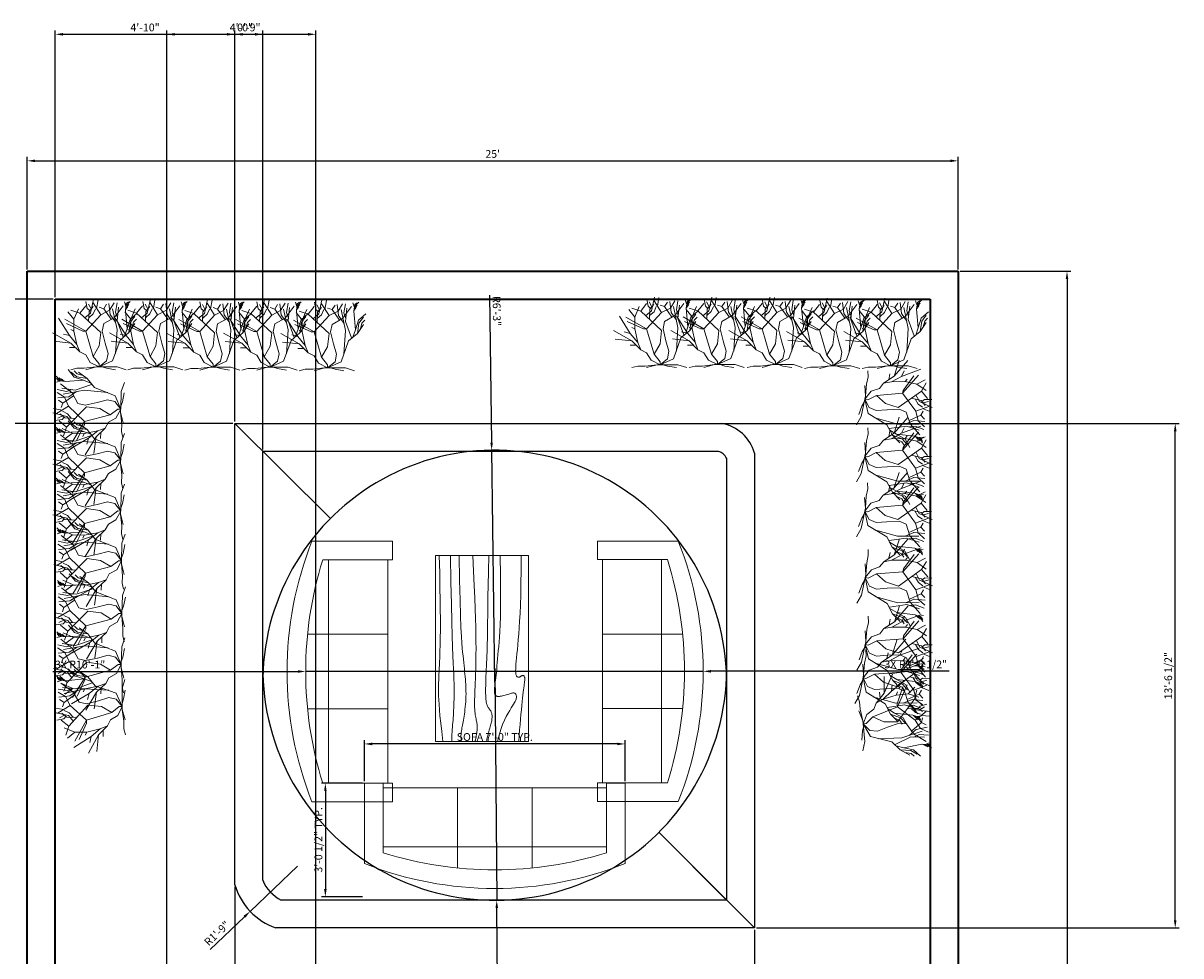
# Model space of a CAD drawing. Units: inches. Extents: x 2318 to 3542, y 1525 to 2117.
# Tile 6 of 6: x 3169 to 3542, y 1816 to 2117. Entities that reach past the tile are written whole.
import ezdxf

# ---------------------------------------------------------------- set-up
doc = ezdxf.new("R2010")
doc.units = ezdxf.units.IN
for name, color, linetype, lineweight in [('A-ANNO-DIMS', 2, 'Continuous', 18), ('A-FLOR', 7, 'Continuous', 25), ('A-FURN', 8, 'Continuous', 18), ('A-WALL', 7, 'Continuous', 35), ('L-PLNT', 94, 'Continuous', 13)]:
    doc.layers.add(name, color=color, linetype=linetype, lineweight=lineweight)
doc.styles.get("Standard").update_dxf_attribs({"font": 'arial.ttf'})
doc.dimstyles.new('ISO-25', dxfattribs={"dimtxt": 2.5, "dimasz": 2.5, "dimexe": 1.25, "dimexo": 0.625, "dimtad": 1, "dimdec": 0, "dimlunit": 3, "dimtxsty": 'Standard', "dimcen": 2.5, "dimadec": 0, "dimazin": 0, "dimtfac": 1, "dimtdec": 0, "dimtmove": 0, "dimatfit": 3, "dimfxl": 1, "dimarcsym": 0})

# ---------------------------------------------------------------- blocks, each defined once
blk = doc.blocks.new('*D19')
at = {"layer": 'A-ANNO-DIMS', "color": 0, "lineweight": -2, "transparency": 16777216}
for p, q in [((3170.43, 2037.71), (3170.43, 2073.97)), ((3172.93, 2072.72), (3467.93, 2072.72)), ((3470.43, 2037.71), (3470.43, 2073.97))]:
    blk.add_line(p, q, dxfattribs=at)
at = {"layer": 'A-ANNO-DIMS', "color": 0, "transparency": 16777216}
for points in [[(3172.93, 2073.14), (3172.93, 2072.3), (3170.43, 2072.72)], [(3467.93, 2073.14), (3467.93, 2072.3), (3470.43, 2072.72)]]:
    blk.add_solid(points, dxfattribs=at)
at = {"layer": 'Defpoints', "color": 0, "transparency": 16777216}
for p in [(3470.43, 2072.72), (3170.43, 2037.09), (3470.43, 2037.09)]:
    blk.add_point(p, dxfattribs=at)
at = {"layer": 'A-ANNO-DIMS', "color": 0, "transparency": 16777216, "insert": (3320.43, 2074.62), "char_height": 2.5, "attachment_point": 5}
blk.add_mtext("25'", dxfattribs=at)
blk = doc.blocks.new('*D20')
at = {"layer": 'A-ANNO-DIMS', "color": 0, "lineweight": -2, "transparency": 16777216}
for p, q in [((3471.06, 2037.09), (3506.78, 2037.09)), ((3505.53, 2034.59), (3505.53, 1559.59)), ((3471.06, 1557.09), (3506.78, 1557.09))]:
    blk.add_line(p, q, dxfattribs=at)
at = {"layer": 'A-ANNO-DIMS', "color": 0, "transparency": 16777216}
for points in [[(3505.11, 2034.59), (3505.94, 2034.59), (3505.53, 2037.09)], [(3505.11, 1559.59), (3505.94, 1559.59), (3505.53, 1557.09)]]:
    blk.add_solid(points, dxfattribs=at)
at = {"layer": 'Defpoints', "color": 0, "transparency": 16777216}
for p in [(3470.43, 2037.09), (3470.43, 1557.09), (3505.53, 1557.09)]:
    blk.add_point(p, dxfattribs=at)
at = {"layer": 'A-ANNO-DIMS', "color": 0, "transparency": 16777216, "insert": (3503.63, 1797.09), "char_height": 2.5, "attachment_point": 5, "rotation": 90}
blk.add_mtext("40'", dxfattribs=at)
blk = doc.blocks.new('*U22')
for p, q in [((-290.3982, 464.5406), (-265.6078, 577.8246)), ((-240.792, 502.285), (-228.3968, 573.8368)), ((-426.72, 414.528), (-475.488, 475.488)), ((-377.952, 463.296), (-451.104, 487.68)), ((-426.72, 414.528), (-390.144, 499.872)), ((-377.952, 463.296), (-329.184, 524.256)), ((-316.7634, 502.285), (-327.6092, 559.9176)), ((-296.5958, 484.4034), (-316.7634, 502.285)), ((-286.512, 498.3226), (-307.4416, 538.0736)), ((-305.8922, 396.9512), (-302.7934, 478.4344)), ((-302.7934, 478.4344), (-270.256, 518.1854)), ((-268.7066, 458.5716), (-250.0884, 500.3038)), ((-207.264, 451.104), (-268.224, 548.64)), ((-182.88, 499.872), (-219.456, 512.064)), ((-207.264, 451.104), (-134.112, 487.68)), ((-182.88, 499.872), (-158.496, 536.448)), ((-121.92, 414.528), (-182.88, 499.872)), ((-129.1844, 450.6214), (-140.0302, 542.036)), ((-134.112, 487.68), (-97.536, 548.64)), ((-73.152, 329.184), (-109.728, 499.872)), ((-97.536, 426.72), (-24.384, 524.256)), ((-85.7758, 472.4908), (-73.3552, 548.005)), ((-73.152, 402.336), (-60.96, 512.064)), ((-12.9032, 555.9552), (-2.0574, 522.1732)), ((-5.1562, 486.3846), (2.5908, 542.036)), ((8.7884, 335.3562), (-5.1562, 486.3846)), ((-3.6068, 492.3536), (14.986, 518.1854)), ((-0.508, 508.254), (22.7584, 536.067)), ((1.0414, 526.1356), (35.1536, 559.9176)), ((2.5908, 542.036), (21.209, 555.9552)), ((-463.296, 280.416), (-552.577, 423.037)), ((-329.184, 316.992), (-499.872, 414.528)), ((-426.72, 316.992), (-426.72, 414.528)), ((-207.264, 304.8), (-377.952, 463.296)), ((-338.455, 424.7896), (-290.3982, 464.5406)), ((-329.184, 316.992), (-207.264, 451.104)), ((-304.3428, 426.7708), (-268.7066, 458.5716)), ((-182.88, 377.952), (-97.536, 426.72)), ((-85.7758, 389.001), (-129.1844, 452.6026)), ((-70.2564, 426.7708), (-85.7758, 472.4908)), ((-24.384, 268.224), (-73.152, 402.336)), ((8.7884, 335.3562), (33.6042, 412.8516)), ((24.384, 304.8), (36.576, 390.144)), ((33.6042, 412.8516), (92.5068, 464.5406)), ((36.576, 390.144), (73.152, 438.912)), ((48.768, 341.376), (60.96, 390.144)), ((60.96, 390.144), (85.344, 414.528)), ((-451.104, 219.456), (-601.0402, 303.8094)), ((-463.296, 280.416), (-512.064, 292.608)), ((-353.568, 316.992), (-487.68, 377.952)), ((-426.72, 316.992), (-451.104, 329.184)), ((-402.336, 207.264), (-426.72, 316.992)), ((-329.184, 316.992), (-353.568, 316.992)), ((-268.224, 109.728), (-329.184, 316.992)), ((-219.456, 195.072), (-207.264, 304.8)), ((-195.072, 316.992), (-182.88, 377.952)), ((-170.688, 219.456), (-195.072, 316.992)), ((-85.344, 134.112), (-73.152, 329.184)), ((-48.768, 243.84), (24.384, 304.8)), ((-12.192, 274.32), (8.7884, 335.3562)), ((24.384, 304.8), (73.152, 377.952)), ((-451.104, 219.456), (-587.4512, 234.2388)), ((-402.336, 207.264), (-463.296, 280.416)), ((-377.952, 146.304), (-451.104, 219.456)), ((-377.952, 146.304), (-402.336, 207.264)), ((-268.224, 109.728), (-219.456, 195.072)), ((-146.304, 134.112), (-170.688, 219.456)), ((-109.728, 73.152), (-48.768, 243.84)), ((-414.528, 182.88), (-463.296, 182.88)), ((-329.184, 121.92), (-377.952, 146.304)), ((-292.608, 60.96), (-329.184, 121.92)), ((-219.456, 48.768), (-268.224, 109.728)), ((-158.496, 73.152), (-146.304, 134.112)), ((-402.336, 12.192), (-451.104, 0)), ((-341.376, 12.192), (-402.336, 12.192)), ((-243.84, 24.384), (-341.376, 12.192)), ((-243.84, 24.384), (-329.184, 0)), ((-219.456, 24.384), (-292.608, 60.96)), ((-243.84, 24.384), (-195.072, 24.384)), ((-219.456, 24.384), (-109.728, 73.152)), ((-219.456, 24.384), (-158.496, 73.152)), ((-219.456, 24.384), (-219.456, 48.768)), ((-219.456, 24.384), (-73.152, 24.384)), ((-195.072, 24.384), (-158.496, 12.192)), ((-158.496, 12.192), (-85.344, 0)), ((-73.152, 24.384), (0, 0))]:
    blk.add_line(p, q)
blk = doc.blocks.new('Table - Rectangular Woodgrain 60 x 30 in.')
for p, q in [((0, 0), (0, -30)), ((60, 0), (0, 0)), ((60, -30), (60, 0)), ((0, -30), (60, -30))]:
    blk.add_line(p, q)
for points in [[(0, -2.4), (4.8155, -2.418), (9.0302, -2.4688), (12.709, -2.5477), (15.9167, -2.65), (18.7181, -2.7711), (21.1781, -2.9063), (23.3616, -3.0508), (25.3333, -3.2), (27.1477, -3.3495), (28.8172, -3.4958), (30.3437, -3.636), (31.7291, -3.7667), (32.9756, -3.8849), (34.0849, -3.9875), (35.059, -4.0714), (35.9, -4.1334), (36.6114, -4.1711), (37.2041, -4.1854), (37.6906, -4.1779), (38.0833, -4.15), (38.3948, -4.1034), (38.6375, -4.0396), (38.8239, -3.9602), (38.9666, -3.8667), (39.0764, -3.7608), (39.1573, -3.6448), (39.2116, -3.521), (39.2416, -3.3917), (39.2498, -3.2593), (39.2385, -3.1261), (39.21, -2.9944), (39.1666, -2.8667), (39.111, -2.7447), (39.0468, -2.6281), (38.978, -2.5163), (38.9083, -2.4083), (38.8418, -2.3035), (38.7823, -2.201), (38.7337, -2.1001), (38.7, -2), (38.6844, -1.9003), (38.6875, -1.8021), (38.7094, -1.707), (38.75, -1.6167), (38.8094, -1.5326), (38.8875, -1.4563), (38.9844, -1.3893), (39.1, -1.3333), (39.2351, -1.2896), (39.3937, -1.2583), (39.5804, -1.2396), (39.8, -1.2333), (40.057, -1.2396), (40.3562, -1.2583), (40.7023, -1.2896), (41.1, -1.3333), (41.5547, -1.3895), (42.0755, -1.4573), (42.6721, -1.5361), (43.3542, -1.625), (44.1316, -1.7233), (45.014, -1.8302), (46.0114, -1.9449), (47.1333, -2.0667), (48.3862, -2.1947), (49.7625, -2.3281), (51.2513, -2.4663), (52.8416, -2.6083), (54.5226, -2.7535), (56.2833, -2.9011), (58.1127, -3.0501), (60, -3.2)], [(0, -9.2), (6.5759, -9.0858), (11.9385, -9.0365), (16.2527, -9.0418), (19.6833, -9.0917), (22.3952, -9.1759), (24.5531, -9.2844), (26.322, -9.4069), (27.8666, -9.5333), (29.3241, -9.6553), (30.7203, -9.7719), (32.0532, -9.8837), (33.3208, -9.9917), (34.5213, -10.0965), (35.6526, -10.199), (36.7128, -10.2999), (37.7, -10.4), (38.6129, -10.4996), (39.4531, -10.5969), (40.223, -10.6895), (40.925, -10.775), (41.5613, -10.8512), (42.1344, -10.9156), (42.6465, -10.966), (43.1, -11), (43.4976, -11.0158), (43.8437, -11.0136), (44.143, -10.9942), (44.4, -10.9583), (44.6195, -10.9069), (44.8062, -10.8406), (44.9648, -10.7603), (45.1, -10.6667), (45.2155, -10.5598), (45.3114, -10.4365), (45.3871, -10.2929), (45.4416, -10.125), (45.4743, -9.929), (45.4844, -9.7011), (45.4709, -9.4371), (45.4333, -9.1333), (45.3716, -8.7883), (45.2896, -8.4104), (45.1919, -8.0107), (45.0833, -7.6), (44.9685, -7.1893), (44.8521, -6.7896), (44.7388, -6.4117), (44.6333, -6.0667), (44.54, -5.7628), (44.4614, -5.4979), (44.4001, -5.2675), (44.3583, -5.0667), (44.3384, -4.8909), (44.3427, -4.7354), (44.3736, -4.5956), (44.4333, -4.4667), (44.5236, -4.3453), (44.6427, -4.2333), (44.7884, -4.1339), (44.9583, -4.05), (45.1501, -3.9849), (45.3614, -3.9417), (45.59, -3.9234), (45.8333, -3.9333), (46.0915, -3.9749), (46.3734, -4.0531), (46.6906, -4.1736), (47.0542, -4.3417), (47.4756, -4.5629), (47.9661, -4.8427), (48.5372, -5.1866), (49.2, -5.6), (49.9676, -6.0844), (50.8594, -6.625), (51.8965, -7.2031), (53.1, -7.8), (54.491, -8.3969), (56.0906, -8.975), (57.9199, -9.5156), (60, -10)], [(0, -12.8), (5.1847, -12.9322), (9.6213, -13.0323), (13.3963, -13.1059), (16.5958, -13.1583), (19.3063, -13.1952), (21.614, -13.2219), (23.6054, -13.2439), (25.3666, -13.2667), (26.9728, -13.2947), (28.4531, -13.3281), (29.8256, -13.3663), (31.1083, -13.4083), (32.3191, -13.4535), (33.476, -13.501), (34.597, -13.5501), (35.7, -13.6), (36.7984, -13.6497), (37.8875, -13.6979), (38.9578, -13.743), (40, -13.7833), (41.0047, -13.8174), (41.9625, -13.8438), (42.864, -13.8607), (43.7, -13.8667), (44.4631, -13.8604), (45.1552, -13.8417), (45.7801, -13.8104), (46.3416, -13.7667), (46.8439, -13.7104), (47.2906, -13.6417), (47.6858, -13.5604), (48.0333, -13.4667), (48.3375, -13.3608), (48.6042, -13.2448), (48.8396, -13.121), (49.05, -12.9917), (49.2417, -12.8593), (49.4208, -12.7261), (49.5937, -12.5944), (49.7667, -12.4667), (49.9452, -12.3451), (50.1323, -12.2313), (50.3303, -12.1268), (50.5416, -12.0333), (50.7686, -11.9524), (51.0135, -11.8854), (51.2788, -11.8341), (51.5666, -11.8), (51.8785, -11.7843), (52.2116, -11.7865), (52.562, -11.8059), (52.926, -11.8417), (53.2998, -11.8931), (53.6795, -11.9594), (54.0614, -12.0397), (54.4416, -12.1333), (54.8223, -12.2401), (55.2293, -12.3625), (55.6942, -12.5037), (56.2489, -12.6667), (56.9251, -12.8547), (57.7545, -13.0708), (58.7689, -13.3182), (60, -13.6)], [(0, -18), (5.124, -17.7273), (9.6609, -17.5057), (13.6705, -17.3303), (17.2125, -17.1958), (20.3467, -17.0973), (23.1328, -17.0297), (25.6307, -16.9878), (27.9, -16.9667), (29.9928, -16.9617), (31.9302, -16.9703), (33.7254, -16.9907), (35.3917, -17.0208), (36.9423, -17.0588), (38.3906, -17.1026), (39.7499, -17.1503), (41.0333, -17.2), (42.2519, -17.2496), (43.4073, -17.2969), (44.4986, -17.3395), (45.525, -17.375), (46.4858, -17.4012), (47.3802, -17.4156), (48.2074, -17.416), (48.9667, -17.4), (49.6583, -17.3662), (50.2872, -17.3167), (50.8595, -17.2547), (51.3812, -17.1833), (51.8584, -17.1057), (52.2971, -17.025), (52.7034, -16.9443), (53.0833, -16.8667), (53.443, -16.7951), (53.789, -16.7313), (54.128, -16.6768), (54.4666, -16.6334), (54.8115, -16.6024), (55.1693, -16.5854), (55.5465, -16.5841), (55.95, -16.6), (56.3828, -16.6337), (56.8346, -16.6823), (57.2915, -16.7418), (57.7396, -16.8084), (58.165, -16.878), (58.5539, -16.9469), (58.8924, -17.0111), (59.1666, -17.0667), (59.3679, -17.1107), (59.5078, -17.1438), (59.6032, -17.1675), (59.6708, -17.1833), (59.7275, -17.193), (59.7901, -17.1979), (59.8753, -17.1998), (60, -17.2)], [(0, -22.4), (8.0098, -22.2501), (14.4094, -22.1011), (19.4168, -21.9535), (23.25, -21.8083), (26.1269, -21.6663), (28.2656, -21.5281), (29.884, -21.3947), (31.2, -21.2667), (32.3967, -21.1448), (33.5172, -21.0292), (34.5697, -20.9198), (35.5625, -20.8167), (36.5037, -20.7198), (37.4015, -20.6292), (38.2642, -20.5448), (39.1, -20.4667), (39.9164, -20.3951), (40.7187, -20.3313), (41.5117, -20.2768), (42.3, -20.2333), (43.0883, -20.2024), (43.8812, -20.1854), (44.6836, -20.1841), (45.5, -20.2), (46.3328, -20.234), (47.1747, -20.2844), (48.0163, -20.3488), (48.8479, -20.425), (49.66, -20.5106), (50.4429, -20.6031), (51.1872, -20.7004), (51.8833, -20.8), (52.5246, -20.8999), (53.1166, -20.9995), (53.6681, -21.0983), (54.1875, -21.1958), (54.6834, -21.2919), (55.1646, -21.3859), (55.6394, -21.4777), (56.1167, -21.5667), (56.6028, -21.6515), (57.0961, -21.7266), (57.5929, -21.7852), (58.0896, -21.8208), (58.5823, -21.8268), (59.0674, -21.7964), (59.5412, -21.723), (60, -21.6)], [(0, -25.2), (8.6355, -25.0504), (15.7026, -24.9031), (21.4049, -24.7606), (25.9458, -24.625), (29.529, -24.4988), (32.3578, -24.3844), (34.6359, -24.284), (36.5667, -24.2), (38.3213, -24.1341), (39.9417, -24.0854), (41.437, -24.0523), (42.8167, -24.0333), (44.0901, -24.0268), (45.2667, -24.0313), (46.3557, -24.0451), (47.3667, -24.0667), (48.309, -24.0947), (49.1928, -24.1287), (50.0284, -24.168), (50.826, -24.2125), (51.5959, -24.2617), (52.3483, -24.3151), (53.0935, -24.3725), (53.8417, -24.4334), (54.6009, -24.497), (55.3699, -24.561), (56.1454, -24.6226), (56.9239, -24.6792), (57.7021, -24.7279), (58.4764, -24.7662), (59.2435, -24.7911), (60, -24.8)], [(0, -28.8), (5.6867, -28.6681), (10.45, -28.5698), (14.407, -28.5012), (17.675, -28.4584), (20.3711, -28.4374), (22.6125, -28.4344), (24.5164, -28.4455), (26.2, -28.4667), (27.762, -28.4947), (29.2276, -28.5281), (30.6033, -28.5663), (31.8958, -28.6084), (33.1118, -28.6535), (34.2578, -28.7011), (35.3405, -28.7501), (36.3666, -28.8), (37.3443, -28.8497), (38.288, -28.8974), (39.2137, -28.9412), (40.1375, -28.9792), (41.0753, -29.0093), (42.0432, -29.0297), (43.0572, -29.0384), (44.1333, -29.0333), (45.2936, -29.0114), (46.5843, -28.9641), (48.0579, -28.8816), (49.7666, -28.7542), (51.7629, -28.5721), (54.0989, -28.3255), (56.8272, -28.0048), (60, -27.6)]]:
    blk.add_lwpolyline(points)
blk = doc.blocks.new('Sofa - Roundback 7 ft.')
for p, q in [((-12.00002, -32.4421), (-12.00003, -6.5971)), ((11.99997, -32.4421), (11.99998, -6.5971)), ((-36.000027, -34), (-36.000027, -11.4696)), ((-35.999844, -13.3819), (35.9998, -13.3819)), ((35.99998, -34), (35.99998, -11.4696)), ((-36.000027, -32.4421), (35.99998, -32.4421))]:
    blk.add_line(p, q)
for points in [[(-36.000027, -34), (-42.000027, -34), (-42.000027, -8)], [(41.99998, -8), (41.99998, -34), (35.99998, -34)]]:
    blk.add_lwpolyline(points)
for centre, radius, start, end in [((0, -114.25), 114.25, 68.43141, 111.5686), ((-0.00001, -127.1968), 121.1968, 72.72033, 107.2797)]:
    blk.add_arc(centre, radius, start, end)
blk = doc.blocks.new('*D38')
at = {"layer": 'A-ANNO-DIMS', "color": 0, "lineweight": -2, "transparency": 16777216}
for p, q in [((3279.1, 1872.73), (3279.1, 1885.95)), ((3360.6, 1884.7), (3281.6, 1884.7)), ((3363.1, 1872.73), (3363.1, 1885.95))]:
    blk.add_line(p, q, dxfattribs=at)
at = {"layer": 'A-ANNO-DIMS', "color": 0, "transparency": 16777216}
for points in [[(3281.6, 1885.12), (3281.6, 1884.28), (3279.1, 1884.7)], [(3360.6, 1885.12), (3360.6, 1884.28), (3363.1, 1884.7)]]:
    blk.add_solid(points, dxfattribs=at)
at = {"layer": 'Defpoints', "color": 0, "transparency": 16777216}
for p in [(3279.1, 1884.7), (3279.1, 1872.1), (3363.1, 1872.1)]:
    blk.add_point(p, dxfattribs=at)
at = {"layer": 'A-ANNO-DIMS', "color": 0, "transparency": 16777216, "insert": (3321.1, 1886.62), "char_height": 2.5, "attachment_point": 5}
blk.add_mtext('SOFA 7\'-0" TYP.', dxfattribs=at)
blk = doc.blocks.new('*D39')
at = {"layer": 'A-ANNO-DIMS', "color": 0, "lineweight": -2, "transparency": 16777216}
for p, q in [((3278.47, 1872.1), (3265.25, 1872.1)), ((3266.5, 1869.6), (3266.5, 1837.93)), ((3278.47, 1835.43), (3265.25, 1835.43))]:
    blk.add_line(p, q, dxfattribs=at)
at = {"layer": 'A-ANNO-DIMS', "color": 0, "transparency": 16777216}
for points in [[(3266.08, 1869.6), (3266.91, 1869.6), (3266.5, 1872.1)], [(3266.08, 1837.93), (3266.91, 1837.93), (3266.5, 1835.43)]]:
    blk.add_solid(points, dxfattribs=at)
at = {"layer": 'Defpoints', "color": 0, "transparency": 16777216}
for p in [(3279.1, 1872.1), (3266.5, 1835.43), (3279.1, 1835.43)]:
    blk.add_point(p, dxfattribs=at)
at = {"layer": 'A-ANNO-DIMS', "color": 0, "transparency": 16777216, "insert": (3264.58, 1853.77), "char_height": 2.5, "attachment_point": 5, "rotation": 90}
blk.add_mtext('3\'-0 1/2" TYP.', dxfattribs=at)
blk = doc.blocks.new('*D53')
at = {"layer": 'A-ANNO-DIMS', "color": 0, "lineweight": -2, "transparency": 16777216}
for p, q in [((3237.33, 1838.64), (3237.33, 1529.19)), ((3404.83, 1824.73), (3404.83, 1529.19)), ((3239.83, 1530.44), (3402.33, 1530.44))]:
    blk.add_line(p, q, dxfattribs=at)
at = {"layer": 'A-ANNO-DIMS', "color": 0, "transparency": 16777216}
for points in [[(3239.83, 1530.86), (3239.83, 1530.02), (3237.33, 1530.44)], [(3402.33, 1530.86), (3402.33, 1530.02), (3404.83, 1530.44)]]:
    blk.add_solid(points, dxfattribs=at)
at = {"layer": 'Defpoints', "color": 0, "transparency": 16777216}
for p in [(3237.33, 1839.27), (3404.83, 1825.36), (3404.83, 1530.44)]:
    blk.add_point(p, dxfattribs=at)
at = {"layer": 'A-ANNO-DIMS', "color": 0, "transparency": 16777216, "insert": (3321.08, 1532.36), "char_height": 2.5, "attachment_point": 5}
blk.add_mtext('13\'-11 1/2"', dxfattribs=at)
blk = doc.blocks.new('*D54')
at = {"layer": 'A-ANNO-DIMS', "color": 0, "lineweight": -2, "transparency": 16777216}
for p, q in [((3237.96, 1988.05), (3541.66, 1988.05)), ((3540.41, 1827.86), (3540.41, 1985.55)), ((3405.46, 1825.36), (3541.66, 1825.36))]:
    blk.add_line(p, q, dxfattribs=at)
at = {"layer": 'A-ANNO-DIMS', "color": 0, "transparency": 16777216}
for points in [[(3539.99, 1985.55), (3540.82, 1985.55), (3540.41, 1988.05)], [(3539.99, 1827.86), (3540.82, 1827.86), (3540.41, 1825.36)]]:
    blk.add_solid(points, dxfattribs=at)
at = {"layer": 'Defpoints', "color": 0, "transparency": 16777216}
for p in [(3237.33, 1988.05), (3540.41, 1988.05), (3404.83, 1825.36)]:
    blk.add_point(p, dxfattribs=at)
at = {"layer": 'A-ANNO-DIMS', "color": 0, "transparency": 16777216, "insert": (3538.49, 1906.7), "char_height": 2.5, "attachment_point": 5, "rotation": 90}
blk.add_mtext('13\'-6 1/2"', dxfattribs=at)
blk = doc.blocks.new('*D55')
at = {"layer": 'A-ANNO-DIMS', "color": 0, "lineweight": -2, "transparency": 16777216}
for p, q in [((3179.43, 2028.71), (3179.43, 2114.76)), ((3181.93, 2113.51), (3234.83, 2113.51)), ((3237.33, 1988.67), (3237.33, 2114.76))]:
    blk.add_line(p, q, dxfattribs=at)
at = {"layer": 'A-ANNO-DIMS', "color": 0, "transparency": 16777216}
for points in [[(3181.93, 2113.93), (3181.93, 2113.1), (3179.43, 2113.51)], [(3234.83, 2113.93), (3234.83, 2113.1), (3237.33, 2113.51)]]:
    blk.add_solid(points, dxfattribs=at)
at = {"layer": 'Defpoints', "color": 0, "transparency": 16777216}
for p in [(3237.33, 2113.51), (3179.43, 2028.09), (3237.33, 1988.05)]:
    blk.add_point(p, dxfattribs=at)
at = {"layer": 'A-ANNO-DIMS', "color": 0, "transparency": 16777216, "insert": (3208.38, 2115.41), "char_height": 2.5, "attachment_point": 5}
blk.add_mtext('4\'-10"', dxfattribs=at)
blk = doc.blocks.new('*D56')
at = {"layer": 'A-ANNO-DIMS', "color": 0, "lineweight": -2, "transparency": 16777216}
for p, q in [((3178.81, 2028.09), (3104.01, 2028.09)), ((3105.26, 2025.59), (3105.26, 1990.55)), ((3236.71, 1988.05), (3104.01, 1988.05))]:
    blk.add_line(p, q, dxfattribs=at)
at = {"layer": 'A-ANNO-DIMS', "color": 0, "transparency": 16777216}
for points in [[(3104.85, 2025.59), (3105.68, 2025.59), (3105.26, 2028.09)], [(3104.85, 1990.55), (3105.68, 1990.55), (3105.26, 1988.05)]]:
    blk.add_solid(points, dxfattribs=at)
at = {"layer": 'Defpoints', "color": 0, "transparency": 16777216}
for p in [(3179.43, 2028.09), (3105.26, 1988.05), (3237.33, 1988.05)]:
    blk.add_point(p, dxfattribs=at)
at = {"layer": 'A-ANNO-DIMS', "color": 0, "transparency": 16777216, "insert": (3103.36, 2008.07), "char_height": 2.5, "attachment_point": 5, "rotation": 90}
blk.add_mtext('3\'-4"', dxfattribs=at)
blk = doc.blocks.new('*D61')
at = {"layer": 'A-ANNO-DIMS', "color": 0, "lineweight": -2, "transparency": 16777216}
for p, q in [((3215.43, 1764.71), (3215.43, 2114.76)), ((3217.93, 2113.51), (3260.93, 2113.51)), ((3263.43, 1764.71), (3263.43, 2114.76))]:
    blk.add_line(p, q, dxfattribs=at)
at = {"layer": 'A-ANNO-DIMS', "color": 0, "transparency": 16777216}
for points in [[(3217.93, 2113.93), (3217.93, 2113.1), (3215.43, 2113.51)], [(3260.93, 2113.93), (3260.93, 2113.1), (3263.43, 2113.51)]]:
    blk.add_solid(points, dxfattribs=at)
at = {"layer": 'Defpoints', "color": 0, "transparency": 16777216}
for p in [(3263.43, 2113.51), (3215.43, 1764.09), (3263.43, 1764.09)]:
    blk.add_point(p, dxfattribs=at)
at = {"layer": 'A-ANNO-DIMS', "color": 0, "transparency": 16777216, "insert": (3239.43, 2115.41), "char_height": 2.5, "attachment_point": 5}
blk.add_mtext('4\'-0"', dxfattribs=at)
blk = doc.blocks.new('*D66')
at = {"layer": 'A-ANNO-DIMS', "color": 0, "lineweight": -2, "transparency": 16777216}
for p, q in [((3237.33, 1988.67), (3237.33, 2114.76)), ((3239.83, 2113.51), (3243.83, 2113.51)), ((3246.33, 1979.67), (3246.33, 2114.76))]:
    blk.add_line(p, q, dxfattribs=at)
at = {"layer": 'A-ANNO-DIMS', "color": 0, "transparency": 16777216}
for points in [[(3239.83, 2113.93), (3239.83, 2113.1), (3237.33, 2113.51)], [(3243.83, 2113.93), (3243.83, 2113.1), (3246.33, 2113.51)]]:
    blk.add_solid(points, dxfattribs=at)
at = {"layer": 'Defpoints', "color": 0, "transparency": 16777216}
for p in [(3246.33, 2113.51), (3237.33, 1988.05), (3246.33, 1979.05)]:
    blk.add_point(p, dxfattribs=at)
at = {"layer": 'A-ANNO-DIMS', "color": 0, "transparency": 16777216, "insert": (3241.83, 2115.41), "char_height": 2.5, "attachment_point": 5}
blk.add_mtext('0\'-9"', dxfattribs=at)
blk = doc.blocks.new('*D75')
at = {"layer": 'A-ANNO-DIMS', "color": 0, "lineweight": -2, "transparency": 16777216}
for p, q in [((3319.43, 2029.38), (3320.06, 1981.88)), ((3321.08, 1904.64), (3320.1, 1979.38))]:
    blk.add_line(p, q, dxfattribs=at)
at = {"layer": 'A-ANNO-DIMS', "color": 0, "transparency": 16777216}
blk.add_solid([(3320.48, 1981.89), (3319.65, 1981.88), (3320.1, 1979.38)], dxfattribs=at)
at = {"layer": 'Defpoints', "color": 0, "transparency": 16777216}
for p in [(3320.1, 1979.38), (3321.08, 1904.64)]:
    blk.add_point(p, dxfattribs=at)
at = {"layer": 'A-ANNO-DIMS', "color": 0, "transparency": 16777216, "insert": (3321.41, 2024.26), "char_height": 2.5, "attachment_point": 5, "rotation": 270.7575}
blk.add_mtext('R6\'-3"', dxfattribs=at)
blk = doc.blocks.new('*D87')
at = {"layer": 'A-ANNO-DIMS', "color": 0, "lineweight": -2, "transparency": 16777216}
for p, q in [((3178.65, 1908.06), (3257.67, 1908.06)), ((3381.37, 1908.06), (3260.17, 1908.06))]:
    blk.add_line(p, q, dxfattribs=at)
at = {"layer": 'A-ANNO-DIMS', "color": 0, "transparency": 16777216}
blk.add_solid([(3257.67, 1908.47), (3257.67, 1907.64), (3260.17, 1908.06)], dxfattribs=at)
at = {"layer": 'Defpoints', "color": 0, "transparency": 16777216}
for p in [(3260.17, 1908.06), (3381.37, 1908.06)]:
    blk.add_point(p, dxfattribs=at)
at = {"layer": 'A-ANNO-DIMS', "color": 0, "transparency": 16777216, "insert": (3187.45, 1909.96), "char_height": 2.5, "attachment_point": 5, "rotation": 0.0002}
blk.add_mtext('3X R10\'-1"', dxfattribs=at)
blk = doc.blocks.new('*D88')
at = {"layer": 'A-ANNO-DIMS', "color": 0, "lineweight": -2, "transparency": 16777216}
for p, q in [((3273.99, 1908.12), (3388.24, 1908.12)), ((3467.54, 1908.12), (3390.74, 1908.12))]:
    blk.add_line(p, q, dxfattribs=at)
at = {"layer": 'A-ANNO-DIMS', "color": 0, "transparency": 16777216}
blk.add_solid([(3390.74, 1908.53), (3390.74, 1907.7), (3388.24, 1908.12)], dxfattribs=at)
at = {"layer": 'Defpoints', "color": 0, "transparency": 16777216}
for p in [(3273.99, 1908.12), (3388.24, 1908.12)]:
    blk.add_point(p, dxfattribs=at)
at = {"layer": 'A-ANNO-DIMS', "color": 0, "transparency": 16777216, "insert": (3456.79, 1910.04), "char_height": 2.5, "attachment_point": 5, "rotation": 359.9998}
blk.add_mtext('3X R9\'-6 1/2"', dxfattribs=at)
blk = doc.blocks.new('*D89')
at = {"layer": 'A-ANNO-DIMS', "color": 0, "lineweight": -2, "transparency": 16777216}
for p, q in [((3257.56, 1845.24), (3242.26, 1830.72)), ((3229.36, 1818.47), (3240.45, 1829))]:
    blk.add_line(p, q, dxfattribs=at)
at = {"layer": 'A-ANNO-DIMS', "color": 0, "transparency": 16777216}
blk.add_solid([(3240.16, 1829.31), (3240.74, 1828.7), (3242.26, 1830.72)], dxfattribs=at)
at = {"layer": 'Defpoints', "color": 0, "transparency": 16777216}
for p in [(3257.56, 1845.24), (3242.26, 1830.72)]:
    blk.add_point(p, dxfattribs=at)
at = {"layer": 'A-ANNO-DIMS', "color": 0, "transparency": 16777216, "insert": (3231.78, 1823.39), "char_height": 2.5, "attachment_point": 5, "rotation": 43.5132}
blk.add_mtext('R1\'-9"', dxfattribs=at)
blk = doc.blocks.new('*D114')
at = {"layer": 'A-ANNO-DIMS', "color": 0, "lineweight": -2, "transparency": 16777216}
for p, q in [((3321.1, 1909.07), (3321.72, 1834.3)), ((3322.14, 1784.3), (3321.74, 1831.8))]:
    blk.add_line(p, q, dxfattribs=at)
at = {"layer": 'A-ANNO-DIMS', "color": 0, "transparency": 16777216}
blk.add_solid([(3322.16, 1831.81), (3321.33, 1831.8), (3321.72, 1834.3)], dxfattribs=at)
at = {"layer": 'Defpoints', "color": 0, "transparency": 16777216}
for p in [(3321.1, 1909.07), (3321.72, 1834.3)]:
    blk.add_point(p, dxfattribs=at)
at = {"layer": 'A-ANNO-DIMS', "color": 0, "transparency": 16777216, "insert": (3324, 1789.46), "char_height": 2.5, "attachment_point": 5, "rotation": 270.4791}
blk.add_mtext('R6\'-3"', dxfattribs=at)

msp = doc.modelspace()

# ---------------------------------------------------------------- linework, layer by layer
at = {"layer": 'A-FLOR'}
for p, q in [((3237.33, 1988.05), (3268.12, 1957.39)), ((3395.83, 1834.36), (3373.98, 1856.21)), ((3373.98, 1856.21), (3404.83, 1825.36))]:
    msp.add_line(p, q, dxfattribs=at)
for points in [[(3237.33, 1839.27), (3237.33, 1988.05), (3394.29, 1988.05)], [(3246.33, 1840.75), (3246.33, 1979.05), (3393.22, 1979.05)], [(3404.83, 1978.49), (3404.83, 1825.36), (3250.54, 1825.36)], [(3395.83, 1976.85), (3395.83, 1834.36), (3252.3, 1834.36)]]:
    msp.add_lwpolyline(points, dxfattribs=at)
for centre, radius, start, end in [((3391.76, 1974.66), 13.62, 16.3159, 79.2827), ((3321.08, 1904.64), 74.76, 0.7415, 180.7733), ((3391.76, 1974.66), 4.62, 28.1949, 71.5513), ((3321.1, 1909.07), 74.77, 179.3603, 1.5978), ((3257.56, 1845.24), 12.09, 201.8112, 244.2237), ((3257.56, 1845.24), 21.09, 196.4709, 250.5551)]:
    msp.add_arc(centre, radius, start, end, dxfattribs=at)
at = {"layer": 'A-WALL'}
for p, q in [((3170.43, 2037.09), (3470.43, 2037.09)), ((3170.43, 1557.09), (3170.43, 2037.09)), ((3470.43, 2037.09), (3470.43, 1557.09)), ((3179.43, 2028.09), (3461.43, 2028.09)), ((3179.43, 1764.09), (3179.43, 2028.09)), ((3461.43, 2028.09), (3461.43, 1764.09))]:
    msp.add_line(p, q, dxfattribs=at)

# ---------------------------------------------------------------- block references
at = {"layer": 'A-FURN'}
for name, p, rotation in [('Sofa - Roundback 7 ft.', (3254.17, 1908.06), 89.99999999999999), ('Sofa - Roundback 7 ft.', (3388.24, 1908.12), 270), ('Table - Rectangular Woodgrain 60 x 30 in.', (3332.01, 1945.49), 270), ('Sofa - Roundback 7 ft.', (3321.1, 1838.1), 180)]:
    msp.add_blockref(name, p, dxfattribs=dict(at, rotation=rotation))
at = {"layer": 'L-PLNT', "xscale": 0.0393700787401575, "yscale": 0.0393700787401575, "zscale": 0.0393700787401575}
for p in [(3202.25, 2005.34), (3220.55, 2005.34), (3238.96, 2005.24), (3257.36, 2005.24), (3275.86, 2005.06), (3383, 2006.03), (3401.47, 2006.06), (3420.21, 2006.06), (3438.73, 2005.71), (3457.25, 2005.71)]:
    msp.add_blockref('*U22', p, dxfattribs=at)
for p, rotation in [((3437.7, 1987.62), 258.2459826834893), ((3201.75, 2001.23), 88.36245576432125), ((3201.75, 1984.76), 88.36245576432125), ((3437.69, 1969.25), 258.2459826834893), ((3437.64, 1951.51), 258.2459826834893), ((3201.75, 1968.41), 88.36245576432125), ((3201.99, 1952.32), 88.36245576432125), ((3437.78, 1930.06), 258.2459826834893), ((3202.13, 1935.37), 88.36245576432125), ((3437.81, 1908.49), 258.2459826834893), ((3201.9, 1918.88), 88.36245576432125), ((3437.09, 1897.7), 258.2459826834893), ((3201.92, 1905.44), 90.4544543415474), ((3439.73, 1882.52), 275.6767207264283)]:
    msp.add_blockref('*U22', p, dxfattribs=dict(at, rotation=rotation))

# ---------------------------------------------------------------- dimensions: what is measured, and where the dimension line sits
at = {"layer": 'A-ANNO-DIMS'}
for base, p1, p2, override, picture, middle in [((3237.33, 2113.51), (3179.43, 2028.09), (3237.33, 1988.05), {"dimdec": 1, "dimlfac": 1, "dimrnd": 0, "dimzin": 1, "dimdsep": 46, "dimlunit": 4, "dimfrac": 2}, '*D55', (3208.38, 2115.41)), ((3263.43, 2113.51), (3215.43, 1764.09), (3263.43, 1764.09), {"dimdec": 1, "dimlfac": 1, "dimrnd": 0, "dimzin": 1, "dimdsep": 46, "dimlunit": 4, "dimfrac": 2}, '*D61', (3239.43, 2115.41)), ((3246.33, 2113.51), (3237.33, 1988.05), (3246.33, 1979.05), {"dimdec": 1, "dimlfac": 1, "dimrnd": 0, "dimzin": 1, "dimdsep": 46, "dimlunit": 4, "dimfrac": 2}, '*D66', (3241.83, 2115.41)), ((3470.43, 2072.72), (3170.43, 2037.09), (3470.43, 2037.09), {"dimclrd": 0, "dimclre": 0, "dimclrt": 0}, '*D19', (3320.43, 2074.62)), ((3404.83, 1530.44), (3237.33, 1839.27), (3404.83, 1825.36), {"dimdec": 1, "dimlfac": 1, "dimrnd": 0, "dimzin": 1, "dimdsep": 46, "dimlunit": 4, "dimfrac": 2}, '*D53', (3321.08, 1532.36))]:
    dim = msp.add_linear_dim(base=base, p1=p1, p2=p2, dimstyle='ISO-25', override=override, dxfattribs=at)
    dim.commit()
    dim.dimension.update_dxf_attribs({"geometry": picture, "text_midpoint": middle})
for base, p1, p2, override, picture, middle in [((3505.53, 1557.09), (3470.43, 2037.09), (3470.43, 1557.09), {"dimclrd": 0, "dimclre": 0, "dimclrt": 0}, '*D20', (3503.63, 1797.09)), ((3105.26, 1988.05), (3179.43, 2028.09), (3237.33, 1988.05), {"dimdec": 1, "dimlfac": 1, "dimrnd": 0, "dimzin": 1, "dimdsep": 46, "dimlunit": 4, "dimfrac": 2}, '*D56', (3103.36, 2008.07)), ((3540.41, 1988.05), (3404.83, 1825.36), (3237.33, 1988.05), {"dimdec": 1, "dimlfac": 1, "dimrnd": 0, "dimzin": 1, "dimdsep": 46, "dimlunit": 4, "dimfrac": 2}, '*D54', (3538.49, 1906.7))]:
    dim = msp.add_linear_dim(base=base, p1=p1, p2=p2, angle=90, dimstyle='ISO-25', override=override, dxfattribs=at)
    dim.commit()
    dim.dimension.update_dxf_attribs({"geometry": picture, "text_midpoint": middle})
for center, mpoint, picture, middle in [((3321.0844, 1904.6352), (3320.096, 1979.3849), '*D75', (3319.503, 2024.2347)), ((3321.1, 1909.07), (3321.72, 1834.3), '*D114', (3322.1, 1789.44)), ((3257.56, 1845.24), (3242.26, 1830.72), '*D89', (3233.09, 1822.01))]:
    dim = msp.add_radius_dim(center=center, mpoint=mpoint, dimstyle='ISO-25', override={"dimdec": 1, "dimlfac": 1, "dimrnd": 0, "dimzin": 1, "dimdsep": 46, "dimlunit": 4, "dimfrac": 2}, dxfattribs=at)
    dim.commit()
    dim.dimension.update_dxf_attribs({"geometry": picture, "text_midpoint": middle, "dimtype": 164})
for center, mpoint, picture, middle in [((3273.99469, 1908.118315), (3388.24469, 1908.118), '*D88', (3456.79469, 1908.117811)), ((3381.37, 1908.06), (3260.17, 1908.06), '*D87', (3187.45, 1908.06))]:
    dim = msp.add_radius_dim(center=center, mpoint=mpoint, text='3X <>', dimstyle='ISO-25', override={"dimdec": 1, "dimlfac": 1, "dimrnd": 0, "dimzin": 1, "dimdsep": 46, "dimlunit": 4, "dimfrac": 2}, dxfattribs=at)
    dim.commit()
    dim.dimension.update_dxf_attribs({"geometry": picture, "text_midpoint": middle, "dimtype": 164})
for base, p1, p2, angle, text, picture, middle in [((3279.1, 1884.7), (3363.1, 1872.1), (3279.1, 1872.1), 180, 'SOFA <> TYP.', '*D38', (3321.1, 1886.62)), ((3266.5, 1835.43), (3279.1, 1872.1), (3279.1, 1835.43), 270, '<> TYP.', '*D39', (3264.58, 1853.77))]:
    dim = msp.add_linear_dim(base=base, p1=p1, p2=p2, angle=angle, text=text, dimstyle='ISO-25', override={"dimdec": 1, "dimlfac": 1, "dimrnd": 0, "dimzin": 1, "dimdsep": 46, "dimlunit": 4, "dimfrac": 2}, dxfattribs=at)
    dim.commit()
    dim.dimension.update_dxf_attribs({"geometry": picture, "text_midpoint": middle})

doc.saveas('drawing.dxf')
